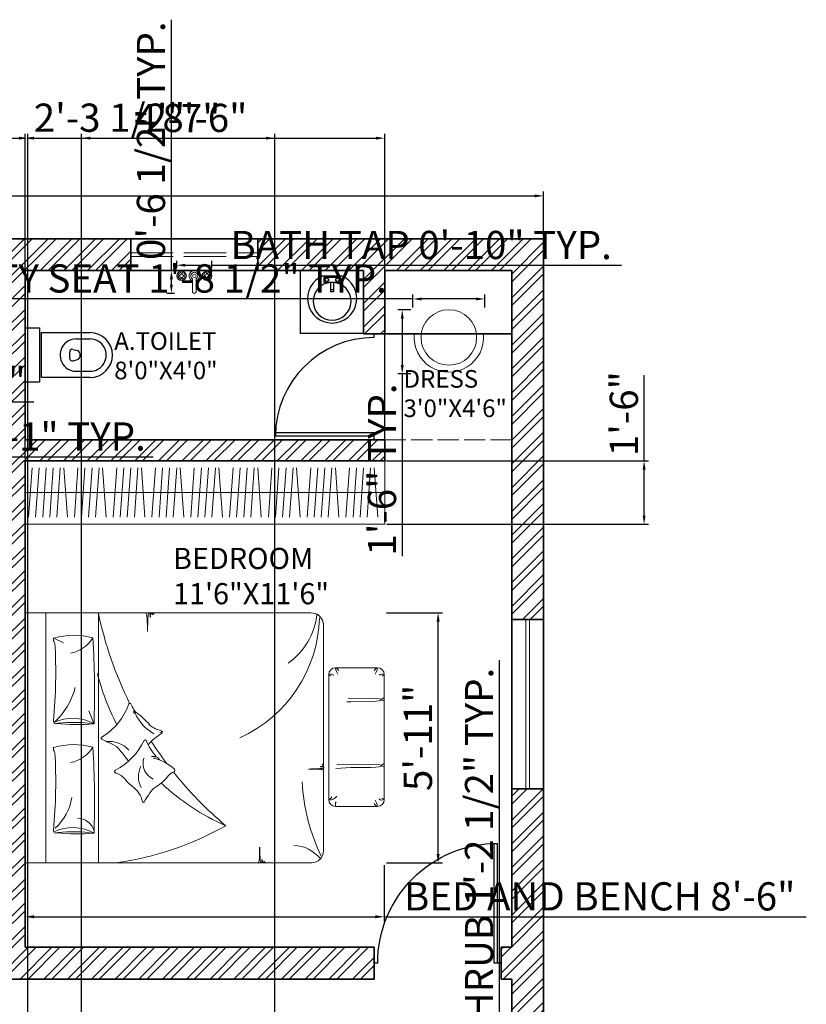
# Model space of a CAD drawing. Units: inches. Extents: x 3595 to 4516, y 2363 to 2965.
# Tile 12 of 12: x 4293 to 4516, y 2686 to 2965. Entities that reach past the tile are written whole.
import ezdxf

# ---------------------------------------------------------------- set-up
doc = ezdxf.new("R2010")
doc.units = ezdxf.units.IN
doc.linetypes.add('ACAD_ISO02W100', pattern=[15, 12, -3])
for name, color, linetype, lineweight in [('A-ANNO-DIMS', 2, 'Continuous', 18), ('A-AREA-IDEN', 7, 'Continuous', 18), ('A-DOOR', 4, 'Continuous', 25), ('A-FLOR-CASE', 9, 'Continuous', 18), ('A-FLOR-FIXT', 8, 'Continuous', 18), ('A-FURN', 43, 'Continuous', 18), ('A-GLAZ', 4, 'Continuous', 18), ('A-GLAZ-HIGH', 4, 'ACAD_ISO02W100', 18), ('A-WALL', 7, 'Continuous', 35), ('A-WALL-OVHD', 7, 'ACAD_ISO02W100', 18)]:
    doc.layers.add(name, color=color, linetype=linetype, lineweight=lineweight)
doc.layers.add('A-WALL-PATT', color=251, linetype='Continuous', lineweight=13, true_color=0x636466)
doc.layers.add('SANTEH', color=7, linetype='Continuous')
doc.styles.get("Standard").update_dxf_attribs({"font": 'arial.ttf'})
doc.dimstyles.new('ISO-25', dxfattribs={"dimtxt": 8, "dimasz": 2.5, "dimexe": 1.25, "dimexo": 0.625, "dimtad": 1, "dimdec": 1, "dimlunit": 3, "dimtxsty": 'Standard', "dimcen": 2.5, "dimadec": 0, "dimazin": 0, "dimtfac": 1, "dimtdec": 1, "dimtmove": 0, "dimatfit": 3, "dimfxl": 1, "dimarcsym": 0})

# ---------------------------------------------------------------- blocks, each defined once
blk = doc.blocks.new('D1')
for p, q in [((1, 0), (1, 34)), ((2, 0), (2, 33.99)), ((0, 0), (2, 0)), ((35, 0), (36, 0))]:
    blk.add_line(p, q)
at = {"ltscale": 0.5}
blk.add_arc((1, 0), 34, 0, 90, dxfattribs=at)
blk = doc.blocks.new('D2')
for p, q in [((1, 0), (1, 28)), ((2, 0), (2, 27.98)), ((0, 0), (2, 0)), ((29, 0), (30, 0))]:
    blk.add_line(p, q)
at = {"ltscale": 0.5}
blk.add_arc((1, 0), 28, 0, 90, dxfattribs=at)
blk = doc.blocks.new('*D5')
at = {"layer": 'A-ANNO-DIMS', "color": 0, "lineweight": -2, "transparency": 16777216}
for p, q in [((4081.24, 2903.67), (4081.24, 2916.47)), ((4441.24, 2903.67), (4441.24, 2916.47)), ((4083.74, 2915.22), (4438.74, 2915.22))]:
    blk.add_line(p, q, dxfattribs=at)
at = {"layer": 'A-ANNO-DIMS', "color": 0, "transparency": 16777216}
for points in [[(4083.74, 2915.63), (4083.74, 2914.8), (4081.24, 2915.22)], [(4438.74, 2915.63), (4438.74, 2914.8), (4441.24, 2915.22)]]:
    blk.add_solid(points, dxfattribs=at)
at = {"layer": 'Defpoints', "color": 0, "transparency": 16777216}
for p in [(4441.24, 2915.22), (4081.24, 2903.04), (4441.24, 2903.04)]:
    blk.add_point(p, dxfattribs=at)
at = {"layer": 'A-ANNO-DIMS', "color": 0, "transparency": 16777216, "insert": (4261.24, 2919.93), "char_height": 8, "attachment_point": 5}
blk.add_mtext("30'", dxfattribs=at)
blk = doc.blocks.new('*X14')
at = {"color": 0}
for p, q in [((3155.9, 8182.9), (3155.9, 8182.9)), ((3147.8, 8143.4), (3147.8, 8143.4)), ((3209.5, 8023.9), (3209.5, 8023.9)), ((3283, 8049.6), (3283, 8049.6)), ((3154.1, 7950.7), (3154.1, 7950.7)), ((3251.6, 7997), (3251.6, 7997))]:
    blk.add_line(p, q, dxfattribs=at)
blk = doc.blocks.new('*X13')
at = {"color": 0}
for p, q in [((3155.9, 8182.9), (3155.9, 8182.9)), ((3139.8, 7939.7), (3139.8, 7939.7))]:
    blk.add_line(p, q, dxfattribs=at)
blk = doc.blocks.new('*X12')
at = {"color": 0}
for p, q in [((3155.9, 8182.9), (3155.9, 8182.9)), ((3139.8, 7939.7), (3139.8, 7939.7))]:
    blk.add_line(p, q, dxfattribs=at)
blk = doc.blocks.new('*X11')
at = {"color": 0}
for p, q in [((3163, 7776.2), (3163, 7776.2)), ((3422.2, 7761.3), (3422.2, 7761.3)), ((3236.2, 7675.7), (3236.2, 7675.7)), ((3244.3, 7698.6), (3244.3, 7698.6)), ((3340.3, 7689.4), (3340.3, 7689.4))]:
    blk.add_line(p, q, dxfattribs=at)
blk = doc.blocks.new('BED1')
for p, q in [((0, -1000), (0, 800)), ((150, 800), (0, 800)), ((150, 800), (150, -1000)), ((2058.7, 800), (150, 800)), ((528, 800), (528, -1000)), ((211.8, 614.9), (277.5, 585.4)), ((2187.2, 354.9), (2187.2, -545.1)), ((2537.2, 404.9), (2237.2, 404.9)), ((2587.2, -545.1), (2587.2, 354.9)), ((2566.3, 178.5), (2565.2, 177.4)), ((2582, 188.1), (2565.4, 174.8)), ((2565.4, 174.8), (2585.7, 165.4)), ((2566.3, -296.8), (2565.2, -297.9)), ((2582, -287.1), (2565.4, -300.5)), ((2565.4, -300.5), (2585.7, -309.9)), ((2237.2, -595.1), (2537.2, -595.1)), ((150, -1000), (0, -1000)), ((150, -1000), (2063.5, -1000))]:
    blk.add_line(p, q)
for points in [[(934, 797.9), (930.9, 797.7), (928.3, 797.4), (926.3, 796.9), (924.9, 796.3), (923.8, 795.6), (923.1, 794.8), (922.7, 793.8), (922.5, 792.7), (922.4, 791.5), (922.5, 790.3), (922.6, 789.2), (922.6, 788.3), (922.6, 787.6), (922.4, 787.3), (922, 787.4), (921.4, 787.9), (920.6, 788.9), (919.5, 790.2), (918.4, 791.6), (917.1, 793.1), (915.9, 794.6), (914.6, 796), (913.3, 797.1), (912.2, 797.9), (911.1, 798.3), (910.1, 798.4), (909.2, 798), (908.3, 797.1), (907.5, 795.8), (906.8, 793.9), (906, 791.4), (905.4, 788.5), (904.8, 785.2), (904.2, 781.7), (903.7, 778.4), (903.2, 775.4), (902.8, 772.9), (902.5, 771.3), (902.3, 770.6), (902.1, 771.2), (902, 772.8), (901.8, 775.2), (901.7, 778.1), (901.5, 781.5), (901.2, 785), (900.8, 788.4), (900.2, 791.5), (899.5, 794.1), (898.6, 796.2), (897.6, 797.9), (896.5, 799.2), (895.3, 800), (894.1, 800.5), (893, 800.7), (891.9, 800.5), (890.9, 800.1), (890, 799), (889.1, 797.1), (888.3, 794), (887.6, 789.3), (886.9, 782.9), (886.2, 774.2), (885.5, 763.1), (884.8, 749.5), (884.2, 734.2), (883.6, 718.3), (883, 702.8), (882.5, 688.8), (882, 677.5), (881.7, 669.8), (881.5, 666.9), (881.3, 669.4), (881.3, 676.7), (881.3, 687.8), (881.2, 701.5), (881.1, 716.8), (880.8, 732.6), (880.2, 748), (879.4, 761.8), (878.3, 773.2), (876.9, 782.2), (875.1, 789.2), (872.9, 794.4), (870.3, 798), (869, 799)], [(2150, -913.5), (2150, 723.2)], [(2327.6, 182.3), (2530, 185.9), (2550.8, 181.9), (2561.7, 179), (2566, 176.7), (2566.9, 174.4), (2566.3, 171.9), (2562, 169.2), (2550.3, 166.5), (2527.7, 163.9), (2490.6, 161.8), (2345.5, 160.2), (2317.8, 158.5)], [(494.7, 3.1), (458.9, 95.3)], [(2149.7, -259.9), (2150, -268.4), (2150.1, -274.1), (2150.1, -278.1), (2150, -281.4), (2149.8, -284), (2149.5, -286.1), (2149.1, -287.8), (2148.7, -289), (2148.1, -289.9), (2147.4, -290.5), (2146.6, -290.8), (2145.6, -291), (2144.6, -291), (2143.6, -291), (2142.7, -290.9), (2141.9, -290.9), (2141.4, -290.9), (2141.1, -291), (2141.2, -291.4), (2141.7, -291.9), (2142.5, -292.6), (2143.5, -293.4), (2144.7, -294.4), (2146, -295.4), (2147.2, -296.5), (2148.4, -297.6), (2149.3, -298.6), (2150, -299.6), (2150.3, -300.5), (2150.4, -301.3), (2150, -302.1), (2149.3, -302.8), (2148.2, -303.5), (2146.6, -304.1), (2144.6, -304.7), (2142.1, -305.2), (2139.3, -305.7), (2136.5, -306.2), (2133.7, -306.6), (2131.2, -307), (2129.2, -307.3), (2127.8, -307.6), (2127.3, -307.8), (2127.7, -308), (2129, -308.1), (2131, -308.2), (2133.5, -308.3), (2136.3, -308.5), (2139.2, -308.7), (2142, -309), (2144.6, -309.5), (2146.8, -310.1), (2148.6, -310.9), (2150, -311.7), (2151, -312.7), (2151.7, -313.6), (2152.1, -314.6), (2152.3, -315.6), (2152.2, -316.5), (2151.8, -317.3), (2150.9, -318.1), (2149.3, -318.8), (2146.7, -319.4), (2142.8, -320), (2137.4, -320.6), (2130.2, -321.2), (2121, -321.8), (2109.7, -322.3), (2096.9, -322.9), (2083.6, -323.4), (2070.7, -323.9), (2059.1, -324.3), (2049.6, -324.7), (2043.2, -325), (2040.8, -325.2), (2042.9, -325.3), (2049, -325.3), (2058.2, -325.3), (2069.6, -325.4), (2082.3, -325.5), (2095.6, -325.8), (2108.4, -326.2), (2119.9, -326.8), (2129.4, -327.8), (2136.9, -329), (2142.7, -330.5), (2147, -332.3), (2150, -334.4), (2150.9, -335.6)], [(2246.5, -294.4), (2530, -289.4), (2550.8, -293.4), (2561.7, -296.3), (2566, -298.6), (2566.9, -300.8), (2566.3, -303.4), (2562, -306.1), (2550.3, -308.8), (2527.7, -311.3), (2490.6, -313.5), (2345.5, -315), (2238.6, -321.8)], [(1733.7, -998.3), (1731.1, -998.1), (1729, -997.8), (1727.4, -997.4), (1726.1, -997), (1725.2, -996.4), (1724.7, -995.7), (1724.3, -994.8), (1724.1, -993.9), (1724.1, -992.9), (1724.1, -991.9), (1724.2, -991), (1724.2, -990.2), (1724.2, -989.7), (1724.1, -989.4), (1723.8, -989.5), (1723.2, -990), (1722.5, -990.8), (1721.7, -991.8), (1720.7, -993), (1719.7, -994.3), (1718.6, -995.5), (1717.5, -996.6), (1716.5, -997.6), (1715.5, -998.3), (1714.6, -998.6), (1713.8, -998.6), (1713, -998.3), (1712.3, -997.6), (1711.7, -996.5), (1711, -994.9), (1710.4, -992.9), (1709.9, -990.4), (1709.4, -987.6), (1708.9, -984.8), (1708.5, -982), (1708.1, -979.5), (1707.8, -977.4), (1707.5, -976.1), (1707.3, -975.5), (1707.1, -976), (1707, -977.3), (1706.9, -979.3), (1706.8, -981.8), (1706.7, -984.6), (1706.4, -987.5), (1706.1, -990.3), (1705.6, -992.9), (1705, -995.1), (1704.2, -996.9), (1703.4, -998.3), (1702.4, -999.3), (1701.5, -1000), (1700.5, -1000.4), (1699.6, -1000.6), (1698.7, -1000.4), (1697.8, -1000.1), (1697, -999.2), (1696.3, -997.6), (1695.7, -995), (1695.1, -991.1), (1694.5, -985.7), (1693.9, -978.5), (1693.3, -969.3), (1692.8, -957.9), (1692.2, -945.2), (1691.7, -931.9), (1691.2, -919), (1690.8, -907.4), (1690.4, -897.9), (1690.1, -891.5), (1689.9, -889.1), (1689.8, -891.2), (1689.8, -897.3), (1689.8, -906.5), (1689.7, -917.9), (1689.6, -930.6), (1689.4, -943.8), (1688.9, -956.6), (1688.3, -968.1), (1687.3, -977.6), (1686.1, -985.2), (1684.6, -991), (1682.8, -995.3), (1680.7, -998.3), (1679.6, -999.2)]]:
    blk.add_lwpolyline(points)
for points in [[(489.2, 619.6, 0.144019), (207.6, 617.9, 0.248643)], [(205.5, 619.6, 0.267769), (215.1, 582.4, -0.037739), (204.3, 21.8, 0.684696), (236.7, 5.5, -0.060702), (497.2, 0.1, -0.046649), (225.9, 3.1, -1.318436)], [(497.2, 0.1, 0.021276), (489.2, 619.6, -0.206383), (326.6, 509.4, 0.237198)], [(211.8, 12.8, 0.143972), (361.6, 262.9, 1.292232)], [(886.4, -150, -0.069098), (985, -66.5, 0.658965), (982.1, -48.7, -0.049789), (927.4, -29, -0.103757), (896.6, -5.4, 0.055725), (800.9, 83.3, -0.11866), (782.7, 104.9, 0.016811), (761.6, 143.9, 0.70791), (748.3, 144, -0.16964), (551.9, -96.6, 0.664036), (554, -110.7, 0.023706), (627, -144.7, -0.134834), (683.2, -188, 0.012748), (746.3, -267.4)], [(969.1, -259.1, 0.263265), (936.3, -236.9, -0.026108), (909.2, -233.2, 0.027613), (945.1, -234.2, -0.089259), (872.7, -120, 0.662242), (857.6, -119.3, -0.162037), (651.8, -332.7, 0.676499), (654, -354.5, -0.160513), (722.9, -401.5, 0.07473), (773.5, -450.3, -0.187721), (845.5, -559.9, 0.70791), (858.8, -561.4, -0.010003), (898.6, -497.3, -0.113819), (947.3, -450.2, 0.099539), (1032.5, -372.4, -0.173425), (1070.9, -346.4, 0.589988), (1076.2, -326.1, 0.137312), (923.9, -245.9, 0.137312)], [(205.5, -168.2, 0.267769), (215.1, -205.4, -0.037739), (204.3, -766, 0.684696), (236.7, -782.3, -0.060702), (497.2, -787.7, -0.046649), (225.9, -784.7, -1.318436)], [(489.2, -168.2, 0.144019), (207.6, -169.9, 0.248643)], [(497.2, -787.7, 0.021276), (489.2, -168.2, -0.206383), (326.6, -278.4, 0.237198)], [(1446, -733.4, -0.095039), (652.8, -1001.7)]]:
    blk.add_lwpolyline(points, format="xyb")
for centre, radius, start, end in [((3208.8, 1363.3), 2739.4, 191.86791, 206.32469), ((1608.1, 842.5), 496.3, 305.19014, 354.02057), ((2062.7, 713.7), 86.5, 0, 93.53765), ((1138.6, 793.9), 983.2, 294.60777, 358.30329), ((2098.7, 754.7), 1625, 193.90497, 207.81692), ((2237.2, 354.9), 50, 90, 180), ((2201.9, 323.3), 34.8, 50.8413, 114.9586), ((2212.2, 381.5), 36.5, 226.80948, 258.3841), ((2321.1, 409.7), 84.5, 185.61958, 217.13957), ((2227.5, 373.5), 32.8, 17.83305, 72.80048), ((2546.9, 373.5), 32.8, 107.19952, 162.16695), ((2453.3, 409.7), 84.5, 322.86043, 354.38042), ((2537.2, 354.9), 50, 0, 90), ((2572.5, 323.3), 34.8, 65.0414, 129.1587), ((2562.2, 381.5), 36.5, 281.6159, 313.19052), ((751.8, 88.7), 34.9, 336.83517, 27.72181), ((684.2, 86), 100.3, 353.675, 10.88198), ((1074.1, 198.8), 306.1, 197.86019, 241.51221), ((341.4, -277.7), 318.5, 60.71255, 115.00895), ((983.7, -79.5), 20.8, 73.79673, 130.45661), ((978.5, -68.6), 14.3, 39.7097, 85.9506), ((602.5, -324), 198.6, 43.20348, 95.05559), ((3208.8, 1363.3), 2739.4, 212.93136, 216.95099), ((981.1, -281.8), 131.1, 164.0372, 243.45361), ((980, -379), 163.4, 152.61037, 209.36102), ((3208.8, 1363.3), 2739.4, 218.63292, 229.94485), ((3402.5, -342.9), 1408.5, 182.99169, 205.68187), ((2098.7, 754.7), 1625, 226.58872, 246.3156), ((-34.4, -471.2), 376.5, 312.01178, 350.96348), ((2178, -513.5), 33, 286.18268, 338.13858), ((2237.2, -545.1), 50, 180, 270), ((2188.1, -476.2), 73, 269.45125, 322.80265), ((2271.1, -580.9), 35.8, 148.90546, 197.55407), ((2453.3, -600), 84.5, 5.61958, 37.13957), ((2537.2, -545.1), 50, 270, 0), ((2572.5, -513.6), 34.8, 230.8413, 294.9586), ((2562.2, -571.8), 36.5, 46.80948, 78.3841), ((2546.9, -563.8), 32.8, 197.83305, 252.80048), ((375.7, -807.4), 128.2, 17.40732, 88.51286), ((341.4, -1065.5), 318.5, 60.71255, 115.00895), ((1929.1, -1126), 250.5, 37.85533, 88.44053), ((2063.5, -913.5), 86.5, 270, 0)]:
    blk.add_arc(centre, radius, start, end)
for name in ['*X13', '*X12', '*X14', '*X11']:
    blk.add_blockref(name, (-2425.3, -8101.4))
blk = doc.blocks.new('AP2041')
blk.add_lwpolyline([(198.4, 175), (248.7, 175, 1.105542), (-248.7, 175), (-198.4, 175)], format="xyb")
blk.add_circle((0, 200), 200)
blk = doc.blocks.new('r11')
at = {"layer": 'SANTEH', "ltscale": 5}
for p, q in [((0, 0), (600, 0)), ((0, -600), (0, 0)), ((600, 0), (600, -600)), ((210.5, -50), (389.5, -50)), ((210.5, -50), (210.5, -50)), ((223.8, -63.2), (376.2, -63.2)), ((223.8, -113.2), (223.8, -63.2)), ((232.7, -78.7), (249.2, -69.1)), ((232.7, -97.7), (232.7, -78.7)), ((249.2, -69.1), (265.7, -78.7)), ((265.7, -78.7), (265.7, -97.7)), ((334.3, -78.7), (350.8, -69.1)), ((334.3, -97.7), (334.3, -78.7)), ((350.8, -69.1), (367.3, -78.7)), ((367.3, -78.7), (367.3, -97.7)), ((376.2, -63.2), (376.2, -113.2)), ((376.2, -113.2), (223.8, -113.2)), ((249.2, -107.2), (232.7, -97.7)), ((265.7, -97.7), (249.2, -107.2)), ((288, -201.6), (288, -113.2)), ((312, -184.3), (288, -184.3)), ((312, -113.2), (312, -201.6)), ((350.8, -107.2), (334.3, -97.7)), ((367.3, -97.7), (350.8, -107.2)), ((312, -201.6), (288, -201.6)), ((600, -600), (0, -600))]:
    blk.add_line(p, q, dxfattribs=at)
for centre, radius, start, end in [((300, -266.2), 234, 112.50001, 67.49999), ((300, -293), 180.2, 93.8183, 86.1817)]:
    blk.add_arc(centre, radius, start, end, dxfattribs=at)
blk = doc.blocks.new('y3')
at = {"layer": 'SANTEH', "ltscale": 5}
for p, q in [((37.5, 130.7), (37.5, 520.7)), ((87.5, 410.7), (87.5, 520.7)), ((346.6, 426.1), (347.5, 520.7)), ((397.5, 520.7), (397.5, 130.7)), ((171.9, 384.5), (181.1, 421.3)), ((263.1, 384.5), (253.9, 421.3)), ((244.3, 357.8), (190.7, 357.8)), ((397.5, 130.7), (37.5, 130.7)), ((67.5, 20.7), (367.5, 20.7))]:
    blk.add_line(p, q, dxfattribs=at)
blk.add_lwpolyline([(0, 115), (435, 115), (435, 0), (0, 0), (0, 115)], dxfattribs=at)
for centre, radius, start, end in [((217.5, 520.7), 180, 0, 180), ((217.5, 520.7), 130, 359.15795, 180), ((217.5, 410.7), 130, 180, 5.98548), ((217.5, 399.9), 42.2, 30.52342, 149.47658), ((190.7, 377.8), 20, 160.50385, 270), ((244.3, 377.8), 20, 270, 19.49615)]:
    blk.add_arc(centre, radius, start, end, dxfattribs=at)
blk = doc.blocks.new('Faucet - Bathroom top')
for p, q in [((-4.107, 0.125), (-4.375, 0.125)), ((-3.75, 0.4788), (-3.75, 0.75)), ((-3.5, 0.482), (-3.5, 0.75)), ((-3.1461, 0.125), (-2.875, 0.125)), ((3.143, 0.125), (2.875, 0.125)), ((3.5, 0.4788), (3.5, 0.75)), ((3.75, 0.482), (3.75, 0.75)), ((4.1039, 0.125), (4.375, 0.125)), ((-4.1039, -0.125), (-4.375, -0.125)), ((-3.75, -0.4821), (-3.75, -0.75)), ((-3.5, -0.4789), (-3.5, -0.75)), ((-3.143, -0.125), (-2.875, -0.125)), ((-0.5, -0.8639), (-0.5, -4.5)), ((0.5, -4.5), (0.5, -0.8631)), ((3.1461, -0.125), (2.875, -0.125)), ((3.5, -0.4821), (3.5, -0.75)), ((3.75, -0.4789), (3.75, -0.75)), ((4.107, -0.125), (4.375, -0.125))]:
    blk.add_line(p, q)
for centre, radius in [((-3.625, 0), 1.375), ((-4.625, 0), 0.2795), ((-3.625, 0), 0.5), ((-3.625, 1), 0.2795), ((-2.625, 0), 0.2795), ((0, 0), 0.5), ((3.625, 0), 1.375), ((2.625, 0), 0.2795), ((3.625, 0), 0.5), ((3.625, 1), 0.2795), ((4.625, 0), 0.2795), ((-3.625, -1), 0.2795), ((3.625, -1), 0.2795)]:
    blk.add_circle(centre, radius)
for centre, radius, start, end in [((-3.625, 0), 1, 105.2407, 164.2093), ((-3.625, 0), 1, 16.44125, 74.07887), ((0, 0), 1.5, 289.6514, 250.3603), ((0, 0), 1, 300.3431, 239.7554), ((3.625, 0), 1, 106.12, 164.0884), ((3.625, 0), 1, 16.23422, 73.90469), ((-3.625, 0), 1, 196.2342, 253.9047), ((-3.625, 0), 1, 286.12, 344.0884), ((3.625, 0), 1, 196.4413, 254.0789), ((3.625, 0), 1, 285.2407, 344.2093), ((0, -4.5), 0.5, 180, 0)]:
    blk.add_arc(centre, radius, start, end)
blk = doc.blocks.new('VENT-GLAZING-36IN')
for p, q in [((0, 1), (36, 1)), ((0, 0), (36, 0))]:
    blk.add_line(p, q)
blk = doc.blocks.new('WIN-GLAZING-48IN')
for p, q in [((0, 1), (48, 1)), ((0, 0), (48, 0))]:
    blk.add_line(p, q)
blk = doc.blocks.new('*D123')
at = {"layer": 'A-ANNO-DIMS', "color": 0, "lineweight": -2, "transparency": 16777216}
for p, q in [((4294.24, 2725.35), (4294.24, 2709.45)), ((4396.1, 2725.35), (4396.1, 2709.45)), ((4296.74, 2710.7), (4393.6, 2710.7)), ((4396.1, 2710.7), (4515.78, 2710.7))]:
    blk.add_line(p, q, dxfattribs=at)
at = {"layer": 'A-ANNO-DIMS', "color": 0, "transparency": 16777216}
for points in [[(4296.74, 2711.12), (4296.74, 2710.28), (4294.24, 2710.7)], [(4393.6, 2711.12), (4393.6, 2710.28), (4396.1, 2710.7)]]:
    blk.add_solid(points, dxfattribs=at)
at = {"layer": 'Defpoints', "color": 0, "transparency": 16777216}
for p in [(4294.24, 2725.98), (4396.1, 2725.98), (4396.1, 2710.7)]:
    blk.add_point(p, dxfattribs=at)
at = {"layer": 'A-ANNO-DIMS', "color": 0, "transparency": 16777216, "insert": (4457.19, 2715.46), "char_height": 8, "attachment_point": 5}
blk.add_mtext('BED AND BENCH 8\'-6"', dxfattribs=at)
blk = doc.blocks.new('*D124')
at = {"layer": 'A-ANNO-DIMS', "color": 0, "lineweight": -2, "transparency": 16777216}
for p, q in [((4396.73, 2796.97), (4412.63, 2796.97)), ((4411.38, 2728.48), (4411.38, 2794.47)), ((4396.73, 2725.98), (4412.63, 2725.98))]:
    blk.add_line(p, q, dxfattribs=at)
at = {"layer": 'A-ANNO-DIMS', "color": 0, "transparency": 16777216}
for points in [[(4410.96, 2794.47), (4411.8, 2794.47), (4411.38, 2796.97)], [(4410.96, 2728.48), (4411.8, 2728.48), (4411.38, 2725.98)]]:
    blk.add_solid(points, dxfattribs=at)
at = {"layer": 'Defpoints', "color": 0, "transparency": 16777216}
for p in [(4396.1, 2796.97), (4411.38, 2796.97), (4396.1, 2725.98)]:
    blk.add_point(p, dxfattribs=at)
at = {"layer": 'A-ANNO-DIMS', "color": 0, "transparency": 16777216, "insert": (4406.67, 2761.47), "char_height": 8, "attachment_point": 5, "rotation": 90}
blk.add_mtext('5\'-11"', dxfattribs=at)
blk = doc.blocks.new('*D125')
at = {"layer": 'A-ANNO-DIMS', "color": 0, "lineweight": -2, "transparency": 16777216}
for p, q in [((4176.58, 2861.74), (4176.58, 2855.55)), ((4213.71, 2861.74), (4213.71, 2855.55)), ((4179.08, 2856.8), (4211.21, 2856.8)), ((4213.71, 2856.8), (4296.71, 2856.8))]:
    blk.add_line(p, q, dxfattribs=at)
at = {"layer": 'A-ANNO-DIMS', "color": 0, "transparency": 16777216}
for points in [[(4179.08, 2857.21), (4179.08, 2856.38), (4176.58, 2856.8)], [(4211.21, 2857.21), (4211.21, 2856.38), (4213.71, 2856.8)]]:
    blk.add_solid(points, dxfattribs=at)
at = {"layer": 'Defpoints', "color": 0, "transparency": 16777216}
for p in [(4176.58, 2862.37), (4213.71, 2862.37), (4213.71, 2856.8)]:
    blk.add_point(p, dxfattribs=at)
at = {"layer": 'A-ANNO-DIMS', "color": 0, "transparency": 16777216, "insert": (4256.46, 2861.56), "char_height": 8, "attachment_point": 5}
blk.add_mtext('DESK SET 3\'-1"', dxfattribs=at)
blk = doc.blocks.new('*D127')
at = {"layer": 'A-ANNO-DIMS', "color": 0, "lineweight": -2, "transparency": 16777216}
for p, q in [((4404.25, 2885.98), (4256.92, 2885.98)), ((4404.25, 2883.56), (4404.25, 2887.23)), ((4422.09, 2885.98), (4406.75, 2885.98)), ((4424.59, 2883.56), (4424.59, 2887.23))]:
    blk.add_line(p, q, dxfattribs=at)
at = {"layer": 'A-ANNO-DIMS', "color": 0, "transparency": 16777216}
for points in [[(4406.75, 2886.4), (4406.75, 2885.57), (4404.25, 2885.98)], [(4422.09, 2886.4), (4422.09, 2885.57), (4424.59, 2885.98)]]:
    blk.add_solid(points, dxfattribs=at)
at = {"layer": 'Defpoints', "color": 0, "transparency": 16777216}
for p in [(4404.25, 2885.98), (4404.25, 2882.93), (4424.59, 2882.93)]:
    blk.add_point(p, dxfattribs=at)
at = {"layer": 'A-ANNO-DIMS', "color": 0, "transparency": 16777216, "insert": (4329.34, 2890.75), "char_height": 8, "attachment_point": 5}
blk.add_mtext('VANITY SEAT 1\'-8 1/2" TYP.', dxfattribs=at)
blk = doc.blocks.new('*D128')
at = {"layer": 'A-ANNO-DIMS', "color": 0, "lineweight": -2, "transparency": 16777216}
for p, q in [((4403.63, 2882.93), (4399.95, 2882.93)), ((4401.2, 2880.43), (4401.2, 2867.22)), ((4403.63, 2864.72), (4399.95, 2864.72)), ((4401.2, 2864.72), (4401.2, 2812.96))]:
    blk.add_line(p, q, dxfattribs=at)
at = {"layer": 'A-ANNO-DIMS', "color": 0, "transparency": 16777216}
for points in [[(4400.79, 2880.43), (4401.62, 2880.43), (4401.2, 2882.93)], [(4400.79, 2867.22), (4401.62, 2867.22), (4401.2, 2864.72)]]:
    blk.add_solid(points, dxfattribs=at)
at = {"layer": 'Defpoints', "color": 0, "transparency": 16777216}
for p in [(4404.25, 2882.93), (4401.2, 2864.72), (4404.25, 2864.72)]:
    blk.add_point(p, dxfattribs=at)
at = {"layer": 'A-ANNO-DIMS', "color": 0, "transparency": 16777216, "insert": (4396.49, 2837.59), "char_height": 8, "attachment_point": 5, "rotation": 90}
blk.add_mtext('1\'-6" TYP.', dxfattribs=at)
blk = doc.blocks.new('*D131')
at = {"layer": 'A-ANNO-DIMS', "color": 0, "lineweight": -2, "transparency": 16777216}
for p, q in [((4231.24, 2844.27), (4231.24, 2839.92)), ((4256.04, 2844.27), (4256.04, 2839.92)), ((4233.74, 2841.17), (4253.54, 2841.17)), ((4256.04, 2841.17), (4330.6, 2841.17))]:
    blk.add_line(p, q, dxfattribs=at)
at = {"layer": 'A-ANNO-DIMS', "color": 0, "transparency": 16777216}
for points in [[(4233.74, 2841.59), (4233.74, 2840.75), (4231.24, 2841.17)], [(4253.54, 2841.59), (4253.54, 2840.75), (4256.04, 2841.17)]]:
    blk.add_solid(points, dxfattribs=at)
at = {"layer": 'Defpoints', "color": 0, "transparency": 16777216}
for p in [(4231.24, 2844.89), (4256.04, 2844.89), (4256.04, 2841.17)]:
    blk.add_point(p, dxfattribs=at)
at = {"layer": 'A-ANNO-DIMS', "color": 0, "transparency": 16777216, "insert": (4294.57, 2845.93), "char_height": 8, "attachment_point": 5}
blk.add_mtext('WC 2\'-1" TYP.', dxfattribs=at)
blk = doc.blocks.new('*D133')
at = {"layer": 'A-ANNO-DIMS', "color": 0, "lineweight": -2, "transparency": 16777216}
for p, q in [((4337.24, 2894.67), (4337.24, 2896.79)), ((4347.24, 2894.67), (4347.24, 2896.79)), ((4339.74, 2895.54), (4344.74, 2895.54)), ((4347.24, 2895.54), (4463.37, 2895.54))]:
    blk.add_line(p, q, dxfattribs=at)
at = {"layer": 'A-ANNO-DIMS', "color": 0, "transparency": 16777216}
for points in [[(4339.74, 2895.96), (4339.74, 2895.13), (4337.24, 2895.54)], [(4344.74, 2895.96), (4344.74, 2895.13), (4347.24, 2895.54)]]:
    blk.add_solid(points, dxfattribs=at)
at = {"layer": 'Defpoints', "color": 0, "transparency": 16777216}
for p in [(4337.24, 2894.04), (4347.24, 2895.54), (4347.24, 2894.04)]:
    blk.add_point(p, dxfattribs=at)
at = {"layer": 'A-ANNO-DIMS', "color": 0, "transparency": 16777216, "insert": (4406.56, 2900.25), "char_height": 8, "attachment_point": 5}
blk.add_mtext('BATH TAP 0\'-10" TYP.', dxfattribs=at)
blk = doc.blocks.new('*D134')
at = {"layer": 'A-ANNO-DIMS', "color": 0, "lineweight": -2, "transparency": 16777216}
for p, q in [((4335.74, 2894.04), (4335.74, 2965.2)), ((4336.62, 2894.04), (4334.49, 2894.04)), ((4335.74, 2890.04), (4335.74, 2891.54)), ((4336.62, 2887.54), (4334.49, 2887.54))]:
    blk.add_line(p, q, dxfattribs=at)
at = {"layer": 'A-ANNO-DIMS', "color": 0, "transparency": 16777216}
for points in [[(4335.33, 2891.54), (4336.16, 2891.54), (4335.74, 2894.04)], [(4335.33, 2890.04), (4336.16, 2890.04), (4335.74, 2887.54)]]:
    blk.add_solid(points, dxfattribs=at)
at = {"layer": 'Defpoints', "color": 0, "transparency": 16777216}
for p in [(4335.74, 2894.04), (4337.24, 2894.04), (4337.24, 2887.54)]:
    blk.add_point(p, dxfattribs=at)
at = {"layer": 'A-ANNO-DIMS', "color": 0, "transparency": 16777216, "insert": (4330.98, 2930.87), "char_height": 8, "attachment_point": 5, "rotation": 90}
blk.add_mtext('0\'-6 1/2" TYP.', dxfattribs=at)
blk = doc.blocks.new('*D143')
at = {"layer": 'A-ANNO-DIMS', "color": 0, "lineweight": -2, "transparency": 16777216}
for p, q in [((4428.78, 2670.16), (4428.78, 2783.51)), ((4427.22, 2670.16), (4430.03, 2670.16)), ((4428.78, 2658.05), (4428.78, 2667.66)), ((4427.22, 2655.55), (4430.03, 2655.55))]:
    blk.add_line(p, q, dxfattribs=at)
at = {"layer": 'A-ANNO-DIMS', "color": 0, "transparency": 16777216}
for points in [[(4428.37, 2667.66), (4429.2, 2667.66), (4428.78, 2670.16)], [(4428.37, 2658.05), (4429.2, 2658.05), (4428.78, 2655.55)]]:
    blk.add_solid(points, dxfattribs=at)
at = {"layer": 'Defpoints', "color": 0, "transparency": 16777216}
for p in [(4426.59, 2670.16), (4428.78, 2670.16), (4426.59, 2655.55)]:
    blk.add_point(p, dxfattribs=at)
at = {"layer": 'A-ANNO-DIMS', "color": 0, "transparency": 16777216, "insert": (4424.02, 2728.08), "char_height": 8, "attachment_point": 5, "rotation": 90}
blk.add_mtext('SHRUB 1\'-2 1/2" TYP.', dxfattribs=at)
blk = doc.blocks.new('*D163')
at = {"layer": 'A-ANNO-DIMS', "color": 0, "lineweight": -2, "transparency": 16777216}
for p, q in [((4267.47, 2626.41), (4267.47, 2932.84)), ((4269.97, 2931.59), (4292.53, 2931.59)), ((4295.03, 2624.44), (4295.03, 2932.84)), ((4295.03, 2931.59), (4338.82, 2931.59))]:
    blk.add_line(p, q, dxfattribs=at)
at = {"layer": 'A-ANNO-DIMS', "color": 0, "transparency": 16777216}
for points in [[(4269.97, 2932.01), (4269.97, 2931.18), (4267.47, 2931.59)], [(4292.53, 2932.01), (4292.53, 2931.18), (4295.03, 2931.59)]]:
    blk.add_solid(points, dxfattribs=at)
at = {"layer": 'Defpoints', "color": 0, "transparency": 16777216}
for p in [(4295.03, 2931.59), (4267.47, 2625.78), (4295.03, 2623.82)]:
    blk.add_point(p, dxfattribs=at)
at = {"layer": 'A-ANNO-DIMS', "color": 0, "transparency": 16777216, "insert": (4318.18, 2936.36), "char_height": 8, "attachment_point": 5}
blk.add_mtext('2\'-3 1/2"', dxfattribs=at)
blk = doc.blocks.new('*D165')
at = {"layer": 'A-ANNO-DIMS', "color": 0, "lineweight": -2, "transparency": 16777216}
for p, q in [((4310.22, 2662.04), (4310.22, 2932.84)), ((4312.72, 2931.59), (4362.53, 2931.59)), ((4365.03, 2662.04), (4365.03, 2932.84))]:
    blk.add_line(p, q, dxfattribs=at)
at = {"layer": 'A-ANNO-DIMS', "color": 0, "transparency": 16777216}
for points in [[(4312.72, 2932.01), (4312.72, 2931.18), (4310.22, 2931.59)], [(4362.53, 2932.01), (4362.53, 2931.18), (4365.03, 2931.59)]]:
    blk.add_solid(points, dxfattribs=at)
at = {"layer": 'Defpoints', "color": 0, "transparency": 16777216}
for p in [(4365.03, 2931.59), (4310.22, 2661.42), (4365.03, 2661.42)]:
    blk.add_point(p, dxfattribs=at)
at = {"layer": 'A-ANNO-DIMS', "color": 0, "transparency": 16777216, "insert": (4337.62, 2936.22), "char_height": 8, "attachment_point": 5}
blk.add_mtext('4\'-7"', dxfattribs=at)
blk = doc.blocks.new('*D168')
at = {"layer": 'A-ANNO-DIMS', "color": 0, "lineweight": -2, "transparency": 16777216}
for p, q in [((4294.24, 2840.67), (4294.24, 2932.84)), ((4296.74, 2931.59), (4393.74, 2931.59)), ((4396.24, 2840.67), (4396.24, 2932.84))]:
    blk.add_line(p, q, dxfattribs=at)
at = {"layer": 'A-ANNO-DIMS', "color": 0, "transparency": 16777216}
for points in [[(4296.74, 2932.01), (4296.74, 2931.18), (4294.24, 2931.59)], [(4393.74, 2932.01), (4393.74, 2931.18), (4396.24, 2931.59)]]:
    blk.add_solid(points, dxfattribs=at)
at = {"layer": 'Defpoints', "color": 0, "transparency": 16777216}
for p in [(4396.24, 2931.59), (4294.24, 2840.04), (4396.24, 2840.04)]:
    blk.add_point(p, dxfattribs=at)
at = {"layer": 'A-ANNO-DIMS', "color": 0, "transparency": 16777216, "insert": (4345.24, 2936.3), "char_height": 8, "attachment_point": 5}
blk.add_mtext('8\'-6"', dxfattribs=at)
blk = doc.blocks.new('*D169')
at = {"layer": 'A-ANNO-DIMS', "color": 0, "lineweight": -2, "transparency": 16777216}
for p, q in [((4469.79, 2840.04), (4469.79, 2864.31)), ((4396.87, 2840.04), (4471.04, 2840.04)), ((4469.79, 2824.54), (4469.79, 2837.54)), ((4396.87, 2822.04), (4471.04, 2822.04))]:
    blk.add_line(p, q, dxfattribs=at)
at = {"layer": 'A-ANNO-DIMS', "color": 0, "transparency": 16777216}
for points in [[(4469.38, 2837.54), (4470.21, 2837.54), (4469.79, 2840.04)], [(4469.38, 2824.54), (4470.21, 2824.54), (4469.79, 2822.04)]]:
    blk.add_solid(points, dxfattribs=at)
at = {"layer": 'Defpoints', "color": 0, "transparency": 16777216}
for p in [(4396.24, 2840.04), (4469.79, 2840.04), (4396.24, 2822.04)]:
    blk.add_point(p, dxfattribs=at)
at = {"layer": 'A-ANNO-DIMS', "color": 0, "transparency": 16777216, "insert": (4465.08, 2853.43), "char_height": 8, "attachment_point": 5, "rotation": 90}
blk.add_mtext('1\'-6"', dxfattribs=at)

msp = doc.modelspace()

# ---------------------------------------------------------------- hatches: boundary and pattern name
at = {"layer": 'A-WALL-PATT'}
h = msp.add_hatch(dxfattribs=at)
h.set_pattern_fill('ANSI32', color=256, scale=0.5)
h.set_pattern_definition([(45, (441.351, 0), (-3.367596, 3.367596), []), (45, (443.596, 0), (-3.367596, 3.367596), [])])
h.paths.add_polyline_path([(4081.24, 2756.04), (4090.24, 2756.04), (4090.24, 2894.04), (4168.24, 2894.04), (4168.24, 2903.04), (4081.24, 2903.04)])
h.paths.add_polyline_path([(4216.24, 2903.04), (4216.24, 2894.04), (4222.24, 2894.04), (4222.24, 2792.04), (4231.24, 2792.04), (4231.24, 2894.04), (4241.74, 2894.04), (4241.74, 2903.04)])
h.paths.add_polyline_path([(4324.24, 2894.04), (4324.24, 2903.04), (4277.74, 2903.04), (4277.74, 2894.04), (4288.24, 2894.04), (4288.24, 2798.04), (4261.24, 2798.04), (4261.24, 2792.04), (4288.24, 2792.04), (4288.24, 2756.04), (4222.24, 2756.04), (4222.24, 2702.04), (4219.24, 2702.04), (4219.24, 2693.04), (4241.74, 2693.04), (4241.74, 2702.04), (4231.24, 2702.04), (4231.24, 2750.04), (4288.24, 2750.04), (4288.24, 2702.04), (4277.74, 2702.04), (4277.74, 2693.04), (4393.24, 2693.04), (4393.24, 2702.04), (4294.24, 2702.04), (4294.24, 2840.04), (4396.24, 2840.04), (4396.24, 2846.04), (4294.24, 2846.04), (4294.24, 2894.04)])
h.paths.add_polyline_path([(4390.24, 2894.04), (4390.24, 2876.04), (4396.24, 2876.04), (4396.24, 2894.04), (4432.24, 2894.04), (4432.24, 2795.04), (4441.24, 2795.04), (4441.24, 2903.04), (4360.24, 2903.04), (4360.24, 2894.04)])
h.paths.add_polyline_path([(4090.24, 2693.04), (4183.24, 2693.04), (4183.24, 2702.04), (4090.24, 2702.04), (4090.24, 2708.04), (4081.24, 2708.04), (4081.24, 2673.54), (4090.24, 2673.54)])
h.paths.add_polyline_path([(4090.24, 2600.04), (4183.24, 2600.04), (4183.24, 2606.04), (4090.24, 2606.04), (4090.24, 2625.54), (4081.24, 2625.54), (4081.24, 2561.04), (4090.24, 2561.04)])
h.paths.add_polyline_path([(4081.24, 2399.04), (4231.24, 2399.04), (4231.24, 2405.04), (4090.24, 2405.04), (4090.24, 2477.04), (4180.24, 2477.04), (4180.24, 2486.04), (4090.24, 2486.04), (4090.24, 2525.04), (4081.24, 2525.04)])
h.paths.add_polyline_path([(4231.24, 2486.04), (4231.24, 2606.04), (4219.24, 2606.04), (4219.24, 2600.04), (4222.24, 2600.04), (4222.24, 2486.04), (4216.24, 2486.04), (4216.24, 2477.04), (4273.24, 2477.04), (4273.24, 2486.04)])
h.paths.add_polyline_path([(4339.24, 2486.04), (4339.24, 2477.04), (4381.24, 2477.04), (4381.24, 2486.04)])
h.paths.add_polyline_path([(4432.24, 2486.04), (4429.24, 2486.04), (4429.24, 2477.04), (4441.24, 2477.04), (4441.24, 2511.54), (4432.24, 2511.54)])
h.paths.add_polyline_path([(4432.24, 2571.54), (4441.24, 2571.54), (4441.24, 2607.54), (4432.24, 2607.54)])
h.paths.add_polyline_path([(4441.24, 2747.04), (4432.24, 2747.04), (4432.24, 2702.04), (4429.24, 2702.04), (4429.24, 2693.04), (4432.24, 2693.04), (4432.24, 2667.54), (4441.24, 2667.54)])

# ---------------------------------------------------------------- linework, layer by layer
at = {"layer": 'A-FLOR-CASE'}
for p, q in [((4296.24, 2838.04), (4295.24, 2824.04)), ((4298.24, 2838.04), (4297.24, 2824.04)), ((4300.24, 2838.04), (4299.24, 2824.04)), ((4302.24, 2838.04), (4301.24, 2824.04)), ((4304.24, 2838.04), (4303.24, 2824.04)), ((4305.24, 2838.04), (4306.24, 2824.04)), ((4309.24, 2838.04), (4308.24, 2824.04)), ((4311.24, 2838.04), (4310.24, 2824.04)), ((4313.24, 2838.04), (4312.24, 2824.04)), ((4315.24, 2838.04), (4314.24, 2824.04)), ((4316.24, 2838.04), (4317.24, 2824.04)), ((4320.24, 2838.04), (4319.24, 2824.04)), ((4322.24, 2838.04), (4321.24, 2824.04)), ((4324.24, 2838.04), (4323.24, 2824.04)), ((4326.24, 2838.04), (4325.24, 2824.04)), ((4327.24, 2838.04), (4328.24, 2824.04)), ((4331.24, 2838.04), (4330.24, 2824.04)), ((4333.24, 2838.04), (4332.24, 2824.04)), ((4335.24, 2838.04), (4334.24, 2824.04)), ((4337.24, 2838.04), (4336.24, 2824.04)), ((4338.24, 2838.04), (4339.24, 2824.04)), ((4342.24, 2838.04), (4341.24, 2824.04)), ((4344.24, 2838.04), (4343.24, 2824.04)), ((4346.24, 2838.04), (4345.24, 2824.04)), ((4348.24, 2838.04), (4347.24, 2824.04)), ((4349.24, 2838.04), (4350.24, 2824.04)), ((4353.24, 2838.04), (4352.24, 2824.04)), ((4355.24, 2838.04), (4354.24, 2824.04)), ((4357.24, 2838.04), (4356.24, 2824.04)), ((4359.24, 2838.04), (4358.24, 2824.04)), ((4360.24, 2838.04), (4361.24, 2824.04)), ((4364.24, 2838.04), (4363.24, 2824.04)), ((4366.24, 2838.04), (4365.24, 2824.04)), ((4368.24, 2838.04), (4367.24, 2824.04)), ((4370.24, 2838.04), (4369.24, 2824.04)), ((4371.24, 2838.04), (4372.24, 2824.04)), ((4375.24, 2838.04), (4374.24, 2824.04)), ((4377.24, 2838.04), (4376.24, 2824.04)), ((4379.24, 2838.04), (4378.24, 2824.04)), ((4381.24, 2838.04), (4380.24, 2824.04)), ((4382.24, 2838.04), (4383.24, 2824.04)), ((4386.24, 2838.04), (4385.24, 2824.04)), ((4388.24, 2838.04), (4387.24, 2824.04)), ((4390.24, 2838.04), (4389.24, 2824.04)), ((4392.24, 2838.04), (4391.24, 2824.04)), ((4393.24, 2838.04), (4394.24, 2824.04)), ((4396.24, 2840.04), (4396.24, 2822.04)), ((4396.24, 2831.04), (4294.24, 2831.04)), ((4294.24, 2822.04), (4396.24, 2822.04))]:
    msp.add_line(p, q, dxfattribs=at)
at = {"layer": 'A-WALL'}
for p, q in [((4324.24, 2894.04), (4324.24, 2903.04)), ((4360.24, 2894.04), (4360.24, 2903.04)), ((4294.24, 2894.04), (4390.24, 2894.04)), ((4294.24, 2894.04), (4294.24, 2846.04)), ((4390.24, 2894.04), (4390.24, 2876.04)), ((4396.24, 2894.04), (4432.24, 2894.04)), ((4396.24, 2894.04), (4396.24, 2876.04)), ((4432.24, 2894.04), (4432.24, 2702.04)), ((4390.24, 2876.04), (4432.24, 2876.04)), ((4294.24, 2846.04), (4396.24, 2846.04)), ((4396.24, 2846.04), (4396.24, 2840.04)), ((4294.24, 2840.04), (4396.24, 2840.04)), ((4294.24, 2840.04), (4294.24, 2702.04)), ((4432.24, 2795.04), (4441.24, 2795.04)), ((4432.24, 2747.04), (4441.24, 2747.04)), ((4294.24, 2702.04), (4393.24, 2702.04)), ((4393.24, 2702.04), (4393.24, 2693.04)), ((4429.24, 2702.04), (4432.24, 2702.04)), ((4429.24, 2702.04), (4429.24, 2693.04)), ((4277.74, 2693.04), (4393.24, 2693.04)), ((4429.24, 2693.04), (4432.24, 2693.04)), ((4432.24, 2693.04), (4432.24, 2486.04))]:
    msp.add_line(p, q, dxfattribs=at)
msp.add_lwpolyline([(4231.24, 2399.04), (4081.24, 2399.04), (4081.24, 2903.04), (4441.24, 2903.04), (4441.24, 2477.04)], dxfattribs=at)
at = {"layer": 'A-WALL-OVHD', "ltscale": 0.5}
for p, q in [((4396.24, 2846.04), (4432.24, 2846.04)), ((4396.24, 2840.04), (4432.24, 2840.04))]:
    msp.add_line(p, q, dxfattribs=at)

# ---------------------------------------------------------------- block references
at = {"layer": 'A-DOOR', "rotation": 90}
msp.add_blockref('D2', (4393.24, 2846.04), dxfattribs=at)
at = {"layer": 'A-DOOR', "xscale": -1}
msp.add_blockref('D1', (4429.24, 2697.54), dxfattribs=at)
at = {"layer": 'A-FLOR-FIXT'}
msp.add_blockref('Faucet - Bathroom top', (4342.24, 2892.54), dxfattribs=at)
at = {"layer": 'A-FLOR-FIXT', "xscale": 0.0297800069284724, "yscale": 0.0297800069284724, "zscale": 0.0297800069284724}
msp.add_blockref('r11', (4372.38, 2894.04), dxfattribs=at)
at = {"layer": 'A-FLOR-FIXT', "xscale": 0.0353848906415677, "yscale": 0.0353848906415677, "zscale": 0.0353848906415677, "rotation": 270}
msp.add_blockref('y3', (4294.24, 2877.74), dxfattribs=at)
at = {"layer": 'A-FURN', "xscale": 0.0393701, "yscale": 0.0393701, "zscale": 0.0393701, "rotation": 180}
msp.add_blockref('AP2041', (4414.42, 2882.93), dxfattribs=at)
at = {"layer": 'A-FURN', "xscale": 0.0393701, "yscale": 0.0393701, "zscale": 0.0393701}
msp.add_blockref('BED1', (4294.24, 2765.41), dxfattribs=at)
at = {"layer": 'A-GLAZ', "rotation": 89.99999999999783}
msp.add_blockref('WIN-GLAZING-48IN', (4437.24, 2747.04), dxfattribs=at)
at = {"layer": 'A-GLAZ-HIGH'}
msp.add_blockref('VENT-GLAZING-36IN', (4324.24, 2898.04), dxfattribs=at)

# ---------------------------------------------------------------- texts
at = {"layer": 'A-AREA-IDEN', "attachment_point": 1}
for s, insert, char_height in [('{\\fTimes New Roman|b0|i0|c0|p18;A.TOILET\\P8\'0"X4\'0"}', (4319.53, 2876.52), 5), ('{\\fTimes New Roman|b0|i0|c0|p18;DRESS\\P3\'0"X4\'6"}', (4401.56, 2865.8), 5), ('{\\fTimes New Roman|b0|i0|c0|p18;BEDROOM\\P11\'6"X11\'6"}', (4336.19, 2815.36), 6)]:
    msp.add_mtext_dynamic_manual_height_columns(s, width=67.3508, gutter_width=12.5, heights=[0], dxfattribs=dict(at, insert=insert, char_height=char_height))

# ---------------------------------------------------------------- dimensions: what is measured, and where the dimension line sits
at = {"layer": 'A-ANNO-DIMS'}
for base, p1, p2, angle, text, picture, middle in [((4335.74, 2894.04), (4337.24, 2887.54), (4337.24, 2894.04), 90, '<> TYP.', '*D134', (4330.98, 2930.87)), ((4404.25, 2885.98), (4424.59, 2882.93), (4404.25, 2882.93), 180, 'VANITY SEAT <> TYP.', '*D127', (4329.34, 2890.75)), ((4401.2, 2864.72), (4404.25, 2882.93), (4404.25, 2864.72), 270, '<> TYP.', '*D128', (4396.49, 2837.59)), ((4428.78, 2670.16), (4426.59, 2655.55), (4426.59, 2670.16), 90, 'SHRUB <> TYP.', '*D143', (4424.02, 2728.08))]:
    dim = msp.add_linear_dim(base=base, p1=p1, p2=p2, angle=angle, text=text, dimstyle='ISO-25', override={"dimdec": 1, "dimlfac": 1, "dimrnd": 0, "dimzin": 1, "dimdsep": 46, "dimlunit": 4, "dimfrac": 2}, dxfattribs=at)
    dim.commit()
    dim.dimension.update_dxf_attribs({"geometry": picture, "text_midpoint": middle})
for base, p1, p2, override, picture, middle in [((4295.03, 2931.59), (4267.47, 2625.78), (4295.03, 2623.82), {"dimdec": 1, "dimlfac": 1, "dimrnd": 0, "dimzin": 1, "dimdsep": 46, "dimlunit": 4, "dimfrac": 2}, '*D163', (4318.18, 2936.36)), ((4396.24, 2931.59), (4294.24, 2840.04), (4396.24, 2840.04), {"dimdec": 1, "dimlfac": 1, "dimrnd": 0, "dimzin": 1, "dimdsep": 46, "dimlunit": 4, "dimfrac": 2}, '*D168', (4345.24, 2936.3)), ((4365.03, 2931.59), (4310.22, 2661.42), (4365.03, 2661.42), {"dimdec": 1, "dimlfac": 1, "dimrnd": 0, "dimzin": 1, "dimdsep": 46, "dimlunit": 4, "dimfrac": 2}, '*D165', (4337.62, 2936.22)), ((4441.24, 2915.22), (4081.24, 2903.04), (4441.24, 2903.04), {"dimclrd": 0, "dimclre": 0, "dimclrt": 0}, '*D5', (4261.24, 2919.93))]:
    dim = msp.add_linear_dim(base=base, p1=p1, p2=p2, dimstyle='ISO-25', override=override, dxfattribs=at)
    dim.commit()
    dim.dimension.update_dxf_attribs({"geometry": picture, "text_midpoint": middle})
for base, p1, p2, text, picture, middle in [((4347.24, 2895.54), (4337.24, 2894.04), (4347.24, 2894.04), 'BATH TAP <> TYP.', '*D133', (4406.56, 2900.25)), ((4213.71, 2856.8), (4176.58, 2862.37), (4213.71, 2862.37), 'DESK SET <>', '*D125', (4256.46, 2861.56)), ((4256.04, 2841.17), (4231.24, 2844.89), (4256.04, 2844.89), 'WC <> TYP.', '*D131', (4294.57, 2845.93)), ((4396.1, 2710.7), (4294.24, 2725.98), (4396.1, 2725.98), 'BED AND BENCH <>', '*D123', (4457.19, 2715.46))]:
    dim = msp.add_linear_dim(base=base, p1=p1, p2=p2, text=text, dimstyle='ISO-25', override={"dimdec": 1, "dimlfac": 1, "dimrnd": 0, "dimzin": 1, "dimdsep": 46, "dimlunit": 4, "dimfrac": 2}, dxfattribs=at)
    dim.commit()
    dim.dimension.update_dxf_attribs({"geometry": picture, "text_midpoint": middle})
for base, p1, p2, picture, middle in [((4469.79, 2840.04), (4396.24, 2822.04), (4396.24, 2840.04), '*D169', (4465.08, 2853.43)), ((4411.38, 2796.97), (4396.1, 2725.98), (4396.1, 2796.97), '*D124', (4406.67, 2761.47))]:
    dim = msp.add_linear_dim(base=base, p1=p1, p2=p2, angle=90, dimstyle='ISO-25', override={"dimdec": 1, "dimlfac": 1, "dimrnd": 0, "dimzin": 1, "dimdsep": 46, "dimlunit": 4, "dimfrac": 2}, dxfattribs=at)
    dim.commit()
    dim.dimension.update_dxf_attribs({"geometry": picture, "text_midpoint": middle})

doc.saveas('drawing.dxf')
